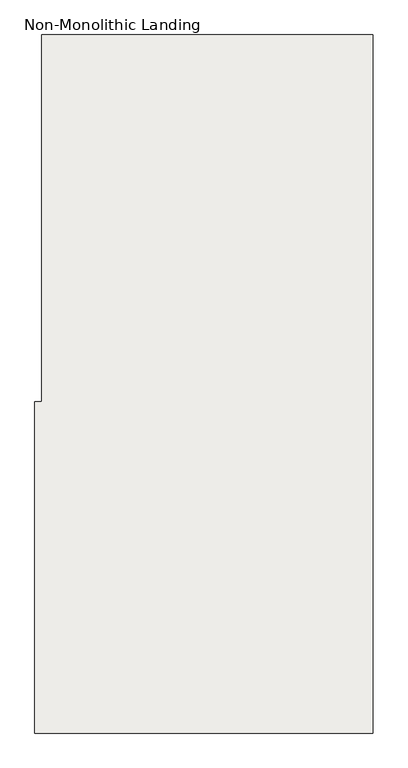
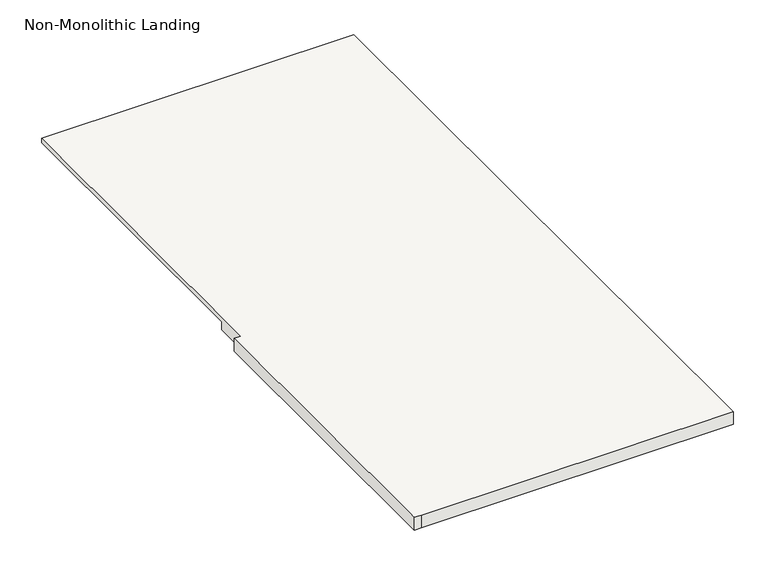
"""IFC4 building model written with IfcOpenShell, lengths in millimetres: slab geometry, Non-Monolithic Landing."""

from ifc_helpers import new_model, si_unit, origin, place, context, project, spatial, faceted_brep, source, transform, mapped, element, save


def non_monolithic_landing_0d67d91a(model_context):
    return source(origin(), model_context, "Body", "Brep", [
        faceted_brep([(-9934.0183666, 3383.7503619, 4711.976087), (-9908.6183666, 3383.7503619, 4686.576087), (-9908.6183666, 2189.9503619, 4686.576087), (-9934.0183666, 2189.9503619, 4711.976087), (-9934.0183666, 2062.9503619, 4731.026087), (-9959.4183666, 2062.9503619, 4731.026087), (-9959.4183666, 869.1503619, 4731.026087), (-9934.0183666, 869.1503619, 4731.026087), (-8740.2183666, 869.1503619, 4731.026087), (-8740.2183666, 3383.7503619, 4731.026087), (-9934.0183666, 3383.7503619, 4731.026087), (-9908.6183666, 2189.9503619, 4680.226087), (-9908.6183666, 3383.7503619, 4680.226087), (-8740.2183666, 3383.7503619, 4680.226087), (-8740.2183666, 869.1503619, 4680.226087), (-9934.0183666, 869.1503619, 4680.226087), (-9959.4183666, 869.1503619, 4680.226087), (-9959.4183666, 2062.9503619, 4680.226087), (-9934.0183666, 2062.9503619, 4680.226087), (-9934.0183666, 2189.9503619, 4680.226087)], [[[0, 1, 2, 3]], [[4, 5, 6, 7, 8, 9, 10]], [[11, 12, 13, 14, 15, 16, 17, 18, 19]], [[12, 11, 2, 1]], [[11, 19, 3, 2]], [[4, 10, 0, 3, 19, 18]], [[5, 4, 18, 17]], [[6, 5, 17, 16]], [[7, 6, 16, 15]], [[8, 7, 15, 14]], [[9, 8, 14, 13]], [[10, 9, 13, 12, 1, 0]]]),
    ])


if __name__ == "__main__":
    model = new_model("IFC4")
    model_context = context("Model", 3, world=origin())
    ifc_project = project(units=[si_unit("LENGTHUNIT", "METRE", prefix="MILLI")], contexts=[model_context])
    site = spatial("IfcSite", under=ifc_project)
    building = spatial("IfcBuilding", under=site)
    placement = place(None, origin())
    non_monolithic_landing_shape = non_monolithic_landing_0d67d91a(model_context)
    element("IfcSlab", 1, ObjectType="Non-Monolithic Landing", at=placement, inside=building, context=model_context, shape_type="MappedRepresentation", body=[
        mapped(non_monolithic_landing_shape, transform((0.0, 0.0, 0.0), x_axis=(1.0, 0.0, 0.0), y_axis=(0.0, 1.0, 0.0), z_axis=(0.0, 0.0, 1.0))),
    ])
    save(model, "model.ifc")
